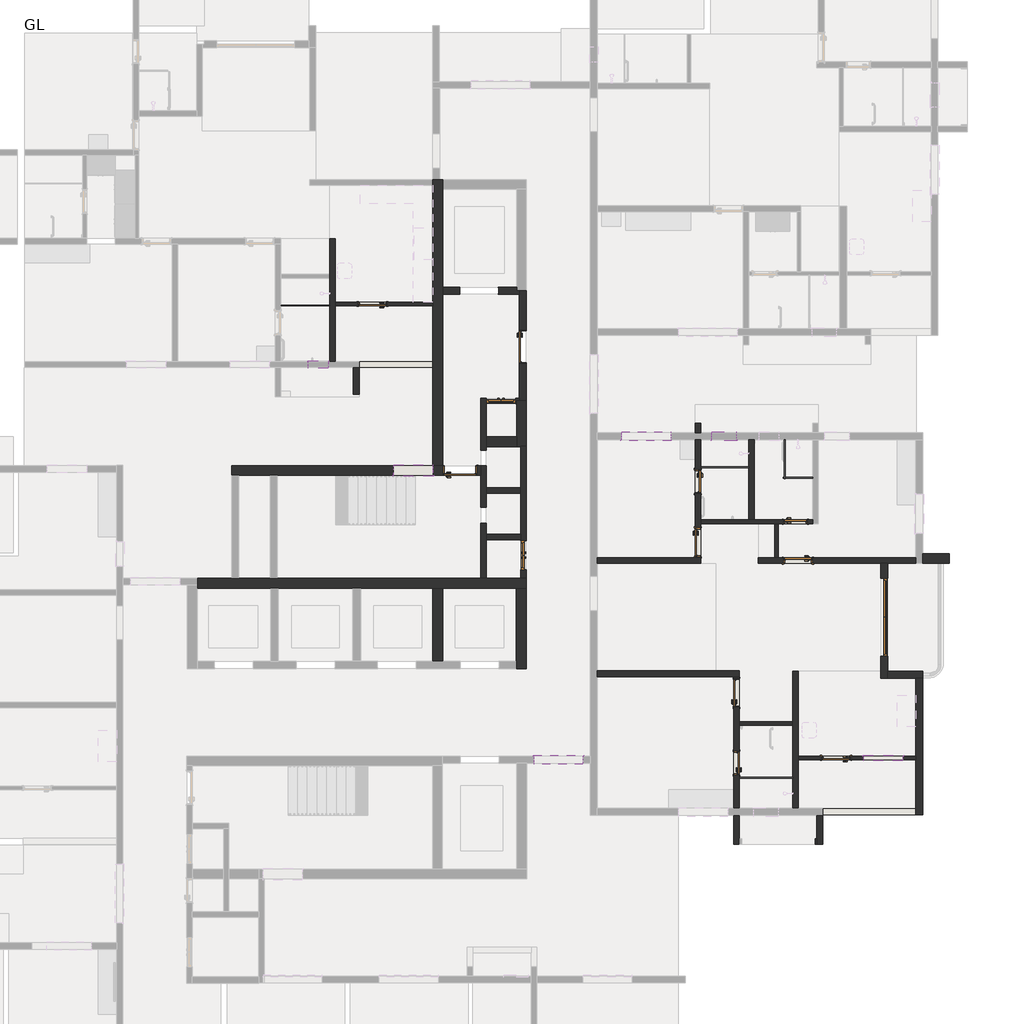
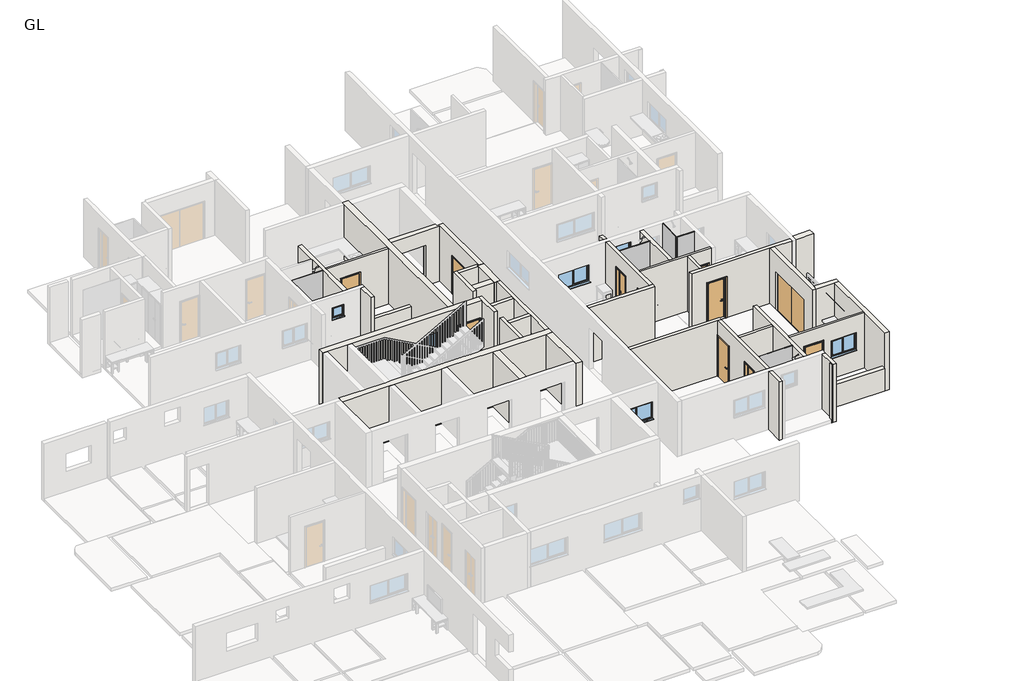
# One storey, part 5 of 14: 39 walls, 13 doors, 6 windows, 5 plates.
# Revit data of these elements (continued)
# Type "Windows_Dbl_Plain : 5'" (continued)
#   Wrap Layers (Int) from Ext = 0.582349 ft
#   Window Board Projection = 0.082021 ft
#   Window Board Extension = 0.082021 ft
#   Visual Light Transmittance = 0.9
#   Solar Heat Gain Coefficient = 0.78
#   Rough Width = 5.0 ft
#   Rough Height = 2.985564 ft
#   Height = 2.985564 ft
#   Width = 5.0 ft
#   Heat Transfer Coefficient (U) = 3.6886 W/(m²·K)
#   Glazing Thickness = 0.07874 ft
#   FrameOffset - External = 0.164042 ft
#   Frame Depth = 0.213255 ft
#   Default Head Height = 6.922572 ft
#   Cill Depth = 0.287073 ft
#   Cavity Closer Width = 0.164042 ft
#   Cavity Closer Offset from Ext = 0.336286 ft
#   Cavity Closer Depth = 0.278871 ft
#   Vis - Cavity Closers = yes
#   Define Thermal Properties by = 1
#   Material Trim = Window Frame
#   Material Glass = Glass
#   Material Frame = Window Frame
#   Wall Closure = (empty or 0)
# Type "Windows_Sgl_Plain : 2'"
#   Type Mark = "60"
#   Operation = "SinglePanel"
#   Construction Type Id = "SGL"
#   Manufacturer = "Revit"
#   Keynote = "L10"
#   Analytic Construction = "Large single-glazed windows"
#   Wrap Layers (Ext) from Ext = 0.336286 ft
#   Wrap Layers (Int) from Ext = 0.582349 ft
#   Window Board Projection = 0.082021 ft
#   Window Board Extension = 0.082021 ft
#   Visual Light Transmittance = 0.9
#   Solar Heat Gain Coefficient = 0.86
#   Rough Width = 2.0 ft
#   Rough Height = 2.0 ft
#   Height = 2.0 ft
#   Width = 2.0 ft
#   Heat Transfer Coefficient (U) = 5.5617 W/(m²·K)
#   Glazing Thickness = 0.07874 ft
#   FrameOffset - External = 0.164042 ft
#   Frame Depth = 0.213255 ft
#   Default Head Height = 6.922572 ft
#   Cill Depth = 0.287073 ft
#   Cavity Closer Width = 0.164042 ft
#   Cavity Closer Offset from Ext = 0.336286 ft
#   Cavity Closer Depth = 0.278871 ft
#   Vis - Cavity Closers = yes
#   Define Thermal Properties by = 1
#   Material Trim = Window Frame
#   Material Glass = Glass
#   Material Frame = Window Frame
#   Wall Closure = (empty or 0)
# Type "Windows_Sgl_Plain : 2.5'"
#   Type Mark = "61"
#   Operation = "SinglePanel"
#   Construction Type Id = "SGL"
#   Manufacturer = "Revit"
#   Keynote = "L10"
#   Analytic Construction = "Large single-glazed windows"
#   Wrap Layers (Ext) from Ext = 0.336286 ft
#   Wrap Layers (Int) from Ext = 0.582349 ft
#   Window Board Projection = 0.082021 ft
#   Window Board Extension = 0.082021 ft
#   Visual Light Transmittance = 0.9
#   Solar Heat Gain Coefficient = 0.86
#   Rough Width = 2.5 ft
#   Rough Height = 2.5 ft
#   Height = 2.5 ft
#   Width = 2.5 ft
#   Heat Transfer Coefficient (U) = 5.5617 W/(m²·K)
#   Glazing Thickness = 0.07874 ft
#   FrameOffset - External = 0.164042 ft
#   Frame Depth = 0.213255 ft
#   Default Head Height = 6.922572 ft
#   Cill Depth = 0.287073 ft
#   Cavity Closer Width = 0.164042 ft
#   Cavity Closer Offset from Ext = 0.336286 ft
#   Cavity Closer Depth = 0.278871 ft
#   Vis - Cavity Closers = yes
#   Define Thermal Properties by = 1
#   Material Trim = Window Frame
#   Material Glass = Glass
#   Material Frame = Window Frame
#   Wall Closure = (empty or 0)
# Element 1 (IfcDoor, "Doors_Concept_ExtDbl : 8'")
#   Phase Created = New Construction
#   Materials on its faces: "Concept", "Door - Glazing"
# Elements 2, 3 (IfcDoor, "Doors_ExtDbl_Flush : 3'")
#   Phase Created = New Construction
#   Materials on its faces: "Door - Handle", "Door - Frame/Mullion", "Door - Panel"
# Elements 4, 5, 6 (IfcDoor, "Doors_IntSgl : 2.5' DOOR")
#   Phase Created = New Construction
#   Materials on its faces: "Door - Architrave", "Door - Handle", "Door - Frame/Mullion (1)", "Door - Panel"
# Elements 7, 8, 9, 10, 11 (IfcDoor, "Doors_IntSgl : 3' DOOR")
#   Phase Created = New Construction
#   Materials on its faces: "Door - Architrave", "Door - Handle", "Door - Frame/Mullion (1)", "Door - Panel"
# Elements 12, 13 (IfcDoor, "Doors_IntSgl : 3.5'")
#   Phase Created = New Construction
#   Materials on its faces: "Door - Architrave", "Door - Handle", "Door - Frame/Mullion (1)", "Door - Panel"
# Elements 14, 15, 16, 17, 18 (IfcPlate, "System Panel : Glazed")
#   Phase Created = New Construction
#   Materials on its faces: "Glass"
# Elements 19, 20, 21, 22, 23, 24, 25, 26, 27, 29, 30, 31, 32, 33, 34, 35, 36, 37, 38 (IfcWall, "W2")
#   Top Offset = 0.0 ft
#   Base Offset = 0.0 ft
#   wall height = 9.84252 ft
#   Phase Created = New Construction
#   Base Constraint = GL
#   Top Constraint = FFL
#   Materials on its faces: "Brick, Common"
# Element 28 (IfcWall, "W2")
#   Top Offset = -6.0 ft
#   Base Offset = 0.0 ft
#   wall height = 3.84252 ft
#   Phase Created = New Construction
#   Base Constraint = GL
#   Top Constraint = FFL
#   Materials on its faces: "Brick, Common"
# Elements 39, 40, 41, 42, 43 (IfcWall, "W3")
#   Top Offset = 0.0 ft
#   Base Offset = 0.0 ft
#   wall height = 9.84252 ft
#   Phase Created = New Construction
#   Base Constraint = GL
#   Top Constraint = FFL
#   Materials on its faces: "Brick, Common"
# Elements 44, 45, 46, 47, 48, 49, 50, 51 (IfcWall, "W4")
#   Top Offset = 0.0 ft
#   Base Offset = 0.0 ft
#   wall height = 9.84252 ft
#   Phase Created = New Construction
#   Base Constraint = GL
#   Top Constraint = FFL
#   Materials on its faces: "Brick, Common"
# Element 52 (IfcWall, "W5")
#   Top Offset = 0.0 ft
#   Base Offset = 0.0 ft
#   wall height = 9.84252 ft
#   Phase Created = New Construction
#   Base Constraint = GL
#   Top Constraint = FFL
#   Materials on its faces: "Brick, Common"
# Element 53 (IfcWall, "W7")
#   Top Offset = 0.0 ft
#   Base Offset = 0.0 ft
#   wall height = 9.84252 ft
#   Phase Created = New Construction
#   Base Constraint = GL
#   Top Constraint = FFL
#   Materials on its faces: "Brick, Common"
# Elements 54, 55, 56 (IfcWall, "W8")
#   Top Offset = 0.0 ft
#   Base Offset = 0.0 ft
#   wall height = 9.84252 ft
#   Phase Created = New Construction
#   Base Constraint = GL
#   Top Constraint = FFL
#   Materials on its faces: "Brick, Common"
# Element 57 (IfcWall, "WALL 1")
#   Top Offset = -6.0 ft
#   Base Offset = 0.0 ft
#   wall height = 3.84252 ft
#   Phase Created = New Construction
#   Base Constraint = GL
#   Top Constraint = FFL
#   Materials on its faces: "Brick, Common"
# Element 58 (IfcWindow, "Windows_Dbl_Plain : 4'")
#   Mark = "57"
#   Phase Created = New Construction
#   Materials on its faces: "Window Frame", "Glass"
# Element 59 (IfcWindow, "Windows_Dbl_Plain : 4'")
#   Mark = "29"
#   Phase Created = New Construction
#   Materials on its faces: "Window Frame", "Glass"
# Element 60 (IfcWindow, "Windows_Dbl_Plain : 5'")
#   Mark = "35"
#   Phase Created = New Construction
#   Materials on its faces: "Window Frame", "Glass"
# Element 61 (IfcWindow, "Windows_Dbl_Plain : 5'")
#   Mark = "26"
#   Phase Created = New Construction
#   Materials on its faces: "Window Frame", "Glass"
# Element 62 (IfcWindow, "Windows_Sgl_Plain : 2'")
#   Mark = "56"
#   Phase Created = New Construction
#   Materials on its faces: "Window Frame", "Glass"
# Element 63 (IfcWindow, "Windows_Sgl_Plain : 2.5'")
#   Mark = "34"
#   Phase Created = New Construction
#   Materials on its faces: "Window Frame", "Glass"
# Materials
#   "Door - Glazing": colour RGB 0 0 255, transparency 0.75
#   "Concept": colour RGB 128 128 255, transparency 0.5
#   "Door - Panel": class "Wood", colour RGB 210 159 95, transparency 0, Keynote = "L20", Cost = 0
#   "Door - Frame/Mullion": class "Wood", colour RGB 212 179 113, transparency 0, Keynote = "L20", Cost = 0
#   "Door - Handle": colour RGB 0 0 0, transparency 0, Keynote = "P21", Cost = 0
#   "Door - Frame/Mullion (1)": class "Wood", colour RGB 212 179 113, transparency 0, Keynote = "L20", Cost = 0
#   "Door - Architrave": class "Wood", colour RGB 154 90 5, transparency 0, Keynote = "P20", Cost = 0
#   "Brick, Common": class "Masonry", colour RGB 170 100 105, transparency 0, Description = "Common brick", Cost = 0
#   "Window Frame": colour RGB 249 249 249, transparency 0, Keynote = "L10", Cost = 0
#   "Glass": class "Glass", colour RGB 0 128 192, transparency 0.9, Description = "Soda Lime Glass", Cost = 0
